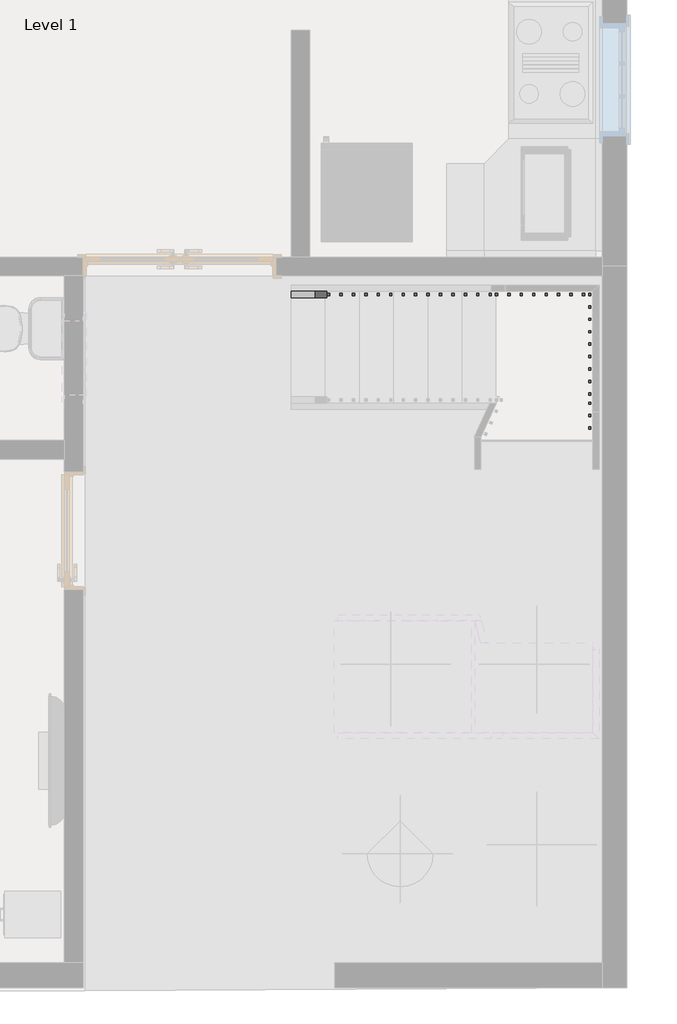
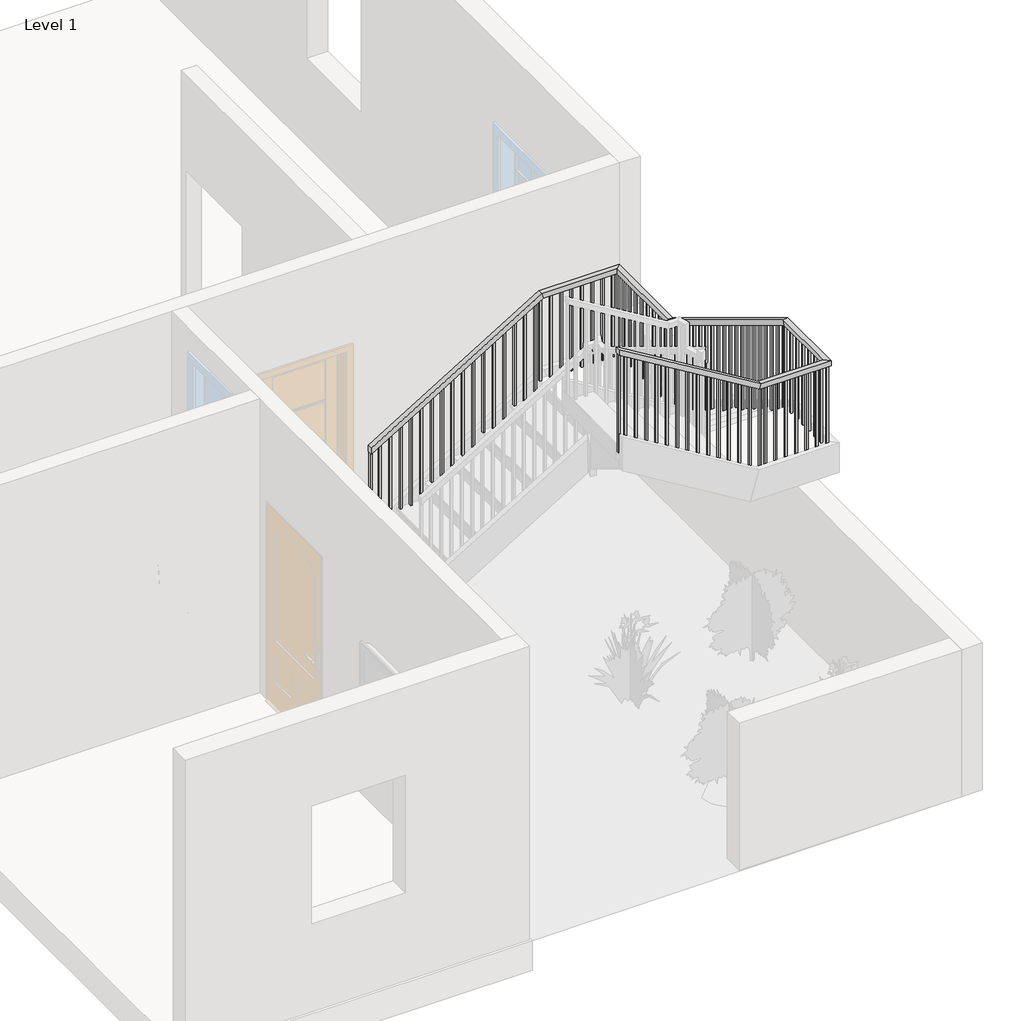
# One storey, part 3 of 4: 1 railing.
"""IFC4 building model written with IfcOpenShell, lengths in millimetres."""

from ifc_helpers import new_model, si_unit, frame, origin, place, context, project, spatial, polyline, outline, extrude, faceted_brep, element, save

model = new_model("IFC4")

# Units and contexts
model_context = context("Model", 3, world=origin())
ifc_project = project(units=[si_unit("LENGTHUNIT", "METRE", prefix="MILLI")], contexts=[model_context])

# Site, building, storey
site = spatial("IfcSite", under=ifc_project)
building = spatial("IfcBuilding", under=site)
storey = spatial("IfcBuildingStorey", under=building, Name="Level 1", Elevation=0.0)

# Railing
placement = place(None, origin())
element("IfcRailing", 1, ObjectType="Handrail - Rectangular", at=placement, inside=storey, context=model_context, shape_type="SolidModel", body=[
    faceted_brep([(-9231.9118598, 5254.5368529, 1083.7333333), (-9231.9118598, 5254.5368529, 1024.3318731), (-9231.9118598, 5203.7368529, 1024.3318731), (-9231.9118598, 5203.7368529, 1083.7333333), (-7555.5118598, 5254.5368529, 2099.7333333), (-7541.3194504, 5254.5368529, 2048.9333333), (-7541.3194504, 5203.7368529, 2048.9333333), (-7555.5118598, 5203.7368529, 2099.7333333), (-6768.1118598, 5254.5368529, 2099.7333333), (-6768.1118598, 5254.5368529, 2048.9333333), (-6818.9118598, 5203.7368529, 2048.9333333), (-6818.9118598, 5203.7368529, 2099.7333333), (-6768.1118598, 4340.1368529, 2099.7333333), (-6768.1118598, 4325.9444434, 2048.9333333), (-6818.9118598, 4325.9444434, 2048.9333333), (-6818.9118598, 4340.1368529, 2099.7333333), (-6768.1118598, 2384.3368529, 3285.0666667), (-6768.1118598, 2370.1444434, 3234.2666667), (-6818.9118598, 2370.1444434, 3234.2666667), (-6818.9118598, 2384.3368529, 3285.0666667), (-6768.1118598, 1647.7368529, 3285.0666667), (-6768.1118598, 1647.7368529, 3234.2666667), (-6818.9118598, 1698.5368529, 3234.2666667), (-6818.9118598, 1698.5368529, 3285.0666667), (-7453.9118598, 1647.7368529, 3285.0666667), (-7468.1042692, 1647.7368529, 3234.2666667), (-7468.1042692, 1698.5368529, 3234.2666667), (-7453.9118598, 1698.5368529, 3285.0666667), (-8850.9118598, 1647.7368529, 4131.7333333), (-8850.9118598, 1698.5368529, 4131.7333333), (-8850.9118598, 1698.5368529, 4072.3318731), (-8850.9118598, 1647.7368529, 4072.3318731)], [[[0, 1, 2, 3]], [[1, 0, 4, 5]], [[2, 1, 5, 6]], [[3, 2, 6, 7]], [[0, 3, 7, 4]], [[5, 4, 8, 9]], [[6, 5, 9, 10]], [[7, 6, 10, 11]], [[4, 7, 11, 8]], [[9, 8, 12, 13]], [[10, 9, 13, 14]], [[11, 10, 14, 15]], [[8, 11, 15, 12]], [[13, 12, 16, 17]], [[14, 13, 17, 18]], [[15, 14, 18, 19]], [[12, 15, 19, 16]], [[17, 16, 20, 21]], [[18, 17, 21, 22]], [[19, 18, 22, 23]], [[16, 19, 23, 20]], [[21, 20, 24, 25]], [[22, 21, 25, 26]], [[23, 22, 26, 27]], [[20, 23, 27, 24]], [[28, 29, 30, 31]], [[25, 24, 28, 31]], [[26, 25, 31, 30]], [[27, 26, 30, 29]], [[24, 27, 29, 28]]]),
    extrude(outline(polyline([(4031.9227822, -8784.2368598), (3048.0, -8784.2368598), (3048.0, -8765.1868598), (4020.3773276, -8765.1868598), (4031.9227822, -8784.2368598)])), frame((0.0, 1663.6118529, 0.0), z_axis=(0.0, 1.0, 0.0), x_axis=(0.0, 0.0, 1.0)), (0.0, 0.0, 1.0), 19.05),
    extrude(outline(polyline([(3970.3470246, -8682.6368598), (3048.0, -8682.6368598), (3048.0, -8663.5868598), (3958.80157, -8663.5868598), (3970.3470246, -8682.6368598)])), frame((0.0, 1663.6118529, 0.0), z_axis=(0.0, 1.0, 0.0), x_axis=(0.0, 0.0, 1.0)), (0.0, 0.0, 1.0), 19.05),
    extrude(outline(polyline([(3908.771267, -8581.0368598), (3048.0, -8581.0368598), (3048.0, -8561.9868598), (3897.2258125, -8561.9868598), (3908.771267, -8581.0368598)])), frame((0.0, 1663.6118529, 0.0), z_axis=(0.0, 1.0, 0.0), x_axis=(0.0, 0.0, 1.0)), (0.0, 0.0, 1.0), 19.05),
    extrude(outline(polyline([(3847.1955094, -8479.4368598), (2878.6666667, -8479.4368598), (2878.6666667, -8460.3868598), (3835.6500549, -8460.3868598), (3847.1955094, -8479.4368598)])), frame((0.0, 1663.6118529, 0.0), z_axis=(0.0, 1.0, 0.0), x_axis=(0.0, 0.0, 1.0)), (0.0, 0.0, 1.0), 19.05),
    extrude(outline(polyline([(3785.6197519, -8377.8368598), (2878.6666667, -8377.8368598), (2878.6666667, -8358.7868598), (3774.0742973, -8358.7868598), (3785.6197519, -8377.8368598)])), frame((0.0, 1663.6118529, 0.0), z_axis=(0.0, 1.0, 0.0), x_axis=(0.0, 0.0, 1.0)), (0.0, 0.0, 1.0), 19.05),
    extrude(outline(polyline([(3724.0439943, -8276.2368598), (2709.3333333, -8276.2368598), (2709.3333333, -8257.1868598), (3712.4985397, -8257.1868598), (3724.0439943, -8276.2368598)])), frame((0.0, 1663.6118529, 0.0), z_axis=(0.0, 1.0, 0.0), x_axis=(0.0, 0.0, 1.0)), (0.0, 0.0, 1.0), 19.05),
    extrude(outline(polyline([(3662.4682367, -8174.6368598), (2709.3333333, -8174.6368598), (2709.3333333, -8155.5868598), (3650.9227822, -8155.5868598), (3662.4682367, -8174.6368598)])), frame((0.0, 1663.6118529, 0.0), z_axis=(0.0, 1.0, 0.0), x_axis=(0.0, 0.0, 1.0)), (0.0, 0.0, 1.0), 19.05),
    extrude(outline(polyline([(3600.8924791, -8073.0368598), (2709.3333333, -8073.0368598), (2709.3333333, -8053.9868598), (3589.3470246, -8053.9868598), (3600.8924791, -8073.0368598)])), frame((0.0, 1663.6118529, 0.0), z_axis=(0.0, 1.0, 0.0), x_axis=(0.0, 0.0, 1.0)), (0.0, 0.0, 1.0), 19.05),
    extrude(outline(polyline([(3539.3167216, -7971.4368598), (2540.0, -7971.4368598), (2540.0, -7952.3868598), (3527.771267, -7952.3868598), (3539.3167216, -7971.4368598)])), frame((0.0, 1663.6118529, 0.0), z_axis=(0.0, 1.0, 0.0), x_axis=(0.0, 0.0, 1.0)), (0.0, 0.0, 1.0), 19.05),
    extrude(outline(polyline([(3477.740964, -7869.8368598), (2540.0, -7869.8368598), (2540.0, -7850.7868598), (3466.1955094, -7850.7868598), (3477.740964, -7869.8368598)])), frame((0.0, 1663.6118529, 0.0), z_axis=(0.0, 1.0, 0.0), x_axis=(0.0, 0.0, 1.0)), (0.0, 0.0, 1.0), 19.05),
    extrude(outline(polyline([(3416.1652064, -7768.2368598), (2540.0, -7768.2368598), (2540.0, -7749.1868598), (3404.6197519, -7749.1868598), (3416.1652064, -7768.2368598)])), frame((0.0, 1663.6118529, 0.0), z_axis=(0.0, 1.0, 0.0), x_axis=(0.0, 0.0, 1.0)), (0.0, 0.0, 1.0), 19.05),
    extrude(outline(polyline([(3354.5894488, -7666.6368598), (2370.6666667, -7666.6368598), (2370.6666667, -7647.5868598), (3343.0439943, -7647.5868598), (3354.5894488, -7666.6368598)])), frame((0.0, 1663.6118529, 0.0), z_axis=(0.0, 1.0, 0.0), x_axis=(0.0, 0.0, 1.0)), (0.0, 0.0, 1.0), 19.05),
    extrude(outline(polyline([(3293.0136913, -7565.0368598), (2370.6666667, -7565.0368598), (2370.6666667, -7545.9868598), (3281.4682367, -7545.9868598), (3293.0136913, -7565.0368598)])), frame((0.0, 1663.6118529, 0.0), z_axis=(0.0, 1.0, 0.0), x_axis=(0.0, 0.0, 1.0)), (0.0, 0.0, 1.0), 19.05),
    extrude(outline(polyline([(-7393.5868598, 1663.6118529), (-7412.6368598, 1663.6118529), (-7412.6368598, 1682.6618529), (-7393.5868598, 1682.6618529), (-7393.5868598, 1663.6118529)])), frame((0.0, 0.0, 2370.6666667), z_axis=(0.0, 0.0, 1.0), x_axis=(1.0, 0.0, 0.0)), (0.0, 0.0, 1.0), 863.6),
    extrude(outline(polyline([(-7291.9868598, 1663.6118529), (-7311.0368598, 1663.6118529), (-7311.0368598, 1682.6618529), (-7291.9868598, 1682.6618529), (-7291.9868598, 1663.6118529)])), frame((0.0, 0.0, 2370.6666667), z_axis=(0.0, 0.0, 1.0), x_axis=(1.0, 0.0, 0.0)), (0.0, 0.0, 1.0), 863.6),
    extrude(outline(polyline([(-7190.3868598, 1663.6118529), (-7209.4368598, 1663.6118529), (-7209.4368598, 1682.6618529), (-7190.3868598, 1682.6618529), (-7190.3868598, 1663.6118529)])), frame((0.0, 0.0, 2370.6666667), z_axis=(0.0, 0.0, 1.0), x_axis=(1.0, 0.0, 0.0)), (0.0, 0.0, 1.0), 863.6),
    extrude(outline(polyline([(-7088.7868598, 1663.6118529), (-7107.8368598, 1663.6118529), (-7107.8368598, 1682.6618529), (-7088.7868598, 1682.6618529), (-7088.7868598, 1663.6118529)])), frame((0.0, 0.0, 2370.6666667), z_axis=(0.0, 0.0, 1.0), x_axis=(1.0, 0.0, 0.0)), (0.0, 0.0, 1.0), 863.6),
    extrude(outline(polyline([(-6987.1868598, 1663.6118529), (-7006.2368598, 1663.6118529), (-7006.2368598, 1682.6618529), (-6987.1868598, 1682.6618529), (-6987.1868598, 1663.6118529)])), frame((0.0, 0.0, 2370.6666667), z_axis=(0.0, 0.0, 1.0), x_axis=(1.0, 0.0, 0.0)), (0.0, 0.0, 1.0), 863.6),
    extrude(outline(polyline([(-6885.5868598, 1663.6118529), (-6904.6368598, 1663.6118529), (-6904.6368598, 1682.6618529), (-6885.5868598, 1682.6618529), (-6885.5868598, 1663.6118529)])), frame((0.0, 0.0, 2370.6666667), z_axis=(0.0, 0.0, 1.0), x_axis=(1.0, 0.0, 0.0)), (0.0, 0.0, 1.0), 863.6),
    extrude(outline(polyline([(-6783.9868598, 1784.2618529), (-6783.9868598, 1765.2118529), (-6803.0368598, 1765.2118529), (-6803.0368598, 1784.2618529), (-6783.9868598, 1784.2618529)])), frame((0.0, 0.0, 2370.6666667), z_axis=(0.0, 0.0, 1.0), x_axis=(1.0, 0.0, 0.0)), (0.0, 0.0, 1.0), 863.6),
    extrude(outline(polyline([(-6783.9868598, 1885.8618529), (-6783.9868598, 1866.8118529), (-6803.0368598, 1866.8118529), (-6803.0368598, 1885.8618529), (-6783.9868598, 1885.8618529)])), frame((0.0, 0.0, 2370.6666667), z_axis=(0.0, 0.0, 1.0), x_axis=(1.0, 0.0, 0.0)), (0.0, 0.0, 1.0), 863.6),
    extrude(outline(polyline([(-6783.9868598, 1987.4618529), (-6783.9868598, 1968.4118529), (-6803.0368598, 1968.4118529), (-6803.0368598, 1987.4618529), (-6783.9868598, 1987.4618529)])), frame((0.0, 0.0, 2370.6666667), z_axis=(0.0, 0.0, 1.0), x_axis=(1.0, 0.0, 0.0)), (0.0, 0.0, 1.0), 863.6),
    extrude(outline(polyline([(-6783.9868598, 2089.0618529), (-6783.9868598, 2070.0118529), (-6803.0368598, 2070.0118529), (-6803.0368598, 2089.0618529), (-6783.9868598, 2089.0618529)])), frame((0.0, 0.0, 2370.6666667), z_axis=(0.0, 0.0, 1.0), x_axis=(1.0, 0.0, 0.0)), (0.0, 0.0, 1.0), 863.6),
    extrude(outline(polyline([(-6783.9868598, 2190.6618529), (-6783.9868598, 2171.6118529), (-6803.0368598, 2171.6118529), (-6803.0368598, 2190.6618529), (-6783.9868598, 2190.6618529)])), frame((0.0, 0.0, 2370.6666667), z_axis=(0.0, 0.0, 1.0), x_axis=(1.0, 0.0, 0.0)), (0.0, 0.0, 1.0), 863.6),
    extrude(outline(polyline([(-6783.9868598, 2292.2618529), (-6783.9868598, 2273.2118529), (-6803.0368598, 2273.2118529), (-6803.0368598, 2292.2618529), (-6783.9868598, 2292.2618529)])), frame((0.0, 0.0, 2370.6666667), z_axis=(0.0, 0.0, 1.0), x_axis=(1.0, 0.0, 0.0)), (0.0, 0.0, 1.0), 863.6),
    extrude(outline(polyline([(2419.2618529, 3204.4985397), (2419.2618529, 2201.3333333), (2400.2118529, 2201.3333333), (2400.2118529, 3216.0439943), (2419.2618529, 3204.4985397)])), frame((-6803.0368598, 0.0, 0.0), z_axis=(1.0, 0.0, 0.0), x_axis=(0.0, 1.0, 0.0)), (0.0, 0.0, 1.0), 19.05),
    extrude(outline(polyline([(2520.8618529, 3142.9227822), (2520.8618529, 2201.3333333), (2501.8118529, 2201.3333333), (2501.8118529, 3154.4682367), (2520.8618529, 3142.9227822)])), frame((-6803.0368598, 0.0, 0.0), z_axis=(1.0, 0.0, 0.0), x_axis=(0.0, 1.0, 0.0)), (0.0, 0.0, 1.0), 19.05),
    extrude(outline(polyline([(2622.4618529, 3081.3470246), (2622.4618529, 2201.3333333), (2603.4118529, 2201.3333333), (2603.4118529, 3092.8924791), (2622.4618529, 3081.3470246)])), frame((-6803.0368598, 0.0, 0.0), z_axis=(1.0, 0.0, 0.0), x_axis=(0.0, 1.0, 0.0)), (0.0, 0.0, 1.0), 19.05),
    extrude(outline(polyline([(2724.0618529, 3019.771267), (2724.0618529, 2032.0), (2705.0118529, 2032.0), (2705.0118529, 3031.3167216), (2724.0618529, 3019.771267)])), frame((-6803.0368598, 0.0, 0.0), z_axis=(1.0, 0.0, 0.0), x_axis=(0.0, 1.0, 0.0)), (0.0, 0.0, 1.0), 19.05),
    extrude(outline(polyline([(2825.6618529, 2958.1955094), (2825.6618529, 2032.0), (2806.6118529, 2032.0), (2806.6118529, 2969.740964), (2825.6618529, 2958.1955094)])), frame((-6803.0368598, 0.0, 0.0), z_axis=(1.0, 0.0, 0.0), x_axis=(0.0, 1.0, 0.0)), (0.0, 0.0, 1.0), 19.05),
    extrude(outline(polyline([(2927.2618529, 2896.6197519), (2927.2618529, 2032.0), (2908.2118529, 2032.0), (2908.2118529, 2908.1652064), (2927.2618529, 2896.6197519)])), frame((-6803.0368598, 0.0, 0.0), z_axis=(1.0, 0.0, 0.0), x_axis=(0.0, 1.0, 0.0)), (0.0, 0.0, 1.0), 19.05),
    extrude(outline(polyline([(3028.8618529, 2835.0439943), (3028.8618529, 1862.6666667), (3009.8118529, 1862.6666667), (3009.8118529, 2846.5894488), (3028.8618529, 2835.0439943)])), frame((-6803.0368598, 0.0, 0.0), z_axis=(1.0, 0.0, 0.0), x_axis=(0.0, 1.0, 0.0)), (0.0, 0.0, 1.0), 19.05),
    extrude(outline(polyline([(3130.4618529, 2773.4682367), (3130.4618529, 1862.6666667), (3111.4118529, 1862.6666667), (3111.4118529, 2785.0136913), (3130.4618529, 2773.4682367)])), frame((-6803.0368598, 0.0, 0.0), z_axis=(1.0, 0.0, 0.0), x_axis=(0.0, 1.0, 0.0)), (0.0, 0.0, 1.0), 19.05),
    extrude(outline(polyline([(3232.0618529, 2711.8924791), (3232.0618529, 1862.6666667), (3213.0118529, 1862.6666667), (3213.0118529, 2723.4379337), (3232.0618529, 2711.8924791)])), frame((-6803.0368598, 0.0, 0.0), z_axis=(1.0, 0.0, 0.0), x_axis=(0.0, 1.0, 0.0)), (0.0, 0.0, 1.0), 19.05),
    extrude(outline(polyline([(3333.6618529, 2650.3167216), (3333.6618529, 1693.3333333), (3314.6118529, 1693.3333333), (3314.6118529, 2661.8621761), (3333.6618529, 2650.3167216)])), frame((-6803.0368598, 0.0, 0.0), z_axis=(1.0, 0.0, 0.0), x_axis=(0.0, 1.0, 0.0)), (0.0, 0.0, 1.0), 19.05),
    extrude(outline(polyline([(3435.2618529, 2588.740964), (3435.2618529, 1693.3333333), (3416.2118529, 1693.3333333), (3416.2118529, 2600.2864185), (3435.2618529, 2588.740964)])), frame((-6803.0368598, 0.0, 0.0), z_axis=(1.0, 0.0, 0.0), x_axis=(0.0, 1.0, 0.0)), (0.0, 0.0, 1.0), 19.05),
    extrude(outline(polyline([(3536.8618529, 2527.1652064), (3536.8618529, 1524.0), (3517.8118529, 1524.0), (3517.8118529, 2538.710661), (3536.8618529, 2527.1652064)])), frame((-6803.0368598, 0.0, 0.0), z_axis=(1.0, 0.0, 0.0), x_axis=(0.0, 1.0, 0.0)), (0.0, 0.0, 1.0), 19.05),
    extrude(outline(polyline([(3638.4618529, 2465.5894488), (3638.4618529, 1524.0), (3619.4118529, 1524.0), (3619.4118529, 2477.1349034), (3638.4618529, 2465.5894488)])), frame((-6803.0368598, 0.0, 0.0), z_axis=(1.0, 0.0, 0.0), x_axis=(0.0, 1.0, 0.0)), (0.0, 0.0, 1.0), 19.05),
    extrude(outline(polyline([(3740.0618529, 2404.0136913), (3740.0618529, 1524.0), (3721.0118529, 1524.0), (3721.0118529, 2415.5591458), (3740.0618529, 2404.0136913)])), frame((-6803.0368598, 0.0, 0.0), z_axis=(1.0, 0.0, 0.0), x_axis=(0.0, 1.0, 0.0)), (0.0, 0.0, 1.0), 19.05),
    extrude(outline(polyline([(3841.6618529, 2342.4379337), (3841.6618529, 1354.6666667), (3822.6118529, 1354.6666667), (3822.6118529, 2353.9833882), (3841.6618529, 2342.4379337)])), frame((-6803.0368598, 0.0, 0.0), z_axis=(1.0, 0.0, 0.0), x_axis=(0.0, 1.0, 0.0)), (0.0, 0.0, 1.0), 19.05),
    extrude(outline(polyline([(3943.2618529, 2280.8621761), (3943.2618529, 1354.6666667), (3924.2118529, 1354.6666667), (3924.2118529, 2292.4076307), (3943.2618529, 2280.8621761)])), frame((-6803.0368598, 0.0, 0.0), z_axis=(1.0, 0.0, 0.0), x_axis=(0.0, 1.0, 0.0)), (0.0, 0.0, 1.0), 19.05),
    extrude(outline(polyline([(4044.8618529, 2219.2864185), (4044.8618529, 1354.6666667), (4025.8118529, 1354.6666667), (4025.8118529, 2230.8318731), (4044.8618529, 2219.2864185)])), frame((-6803.0368598, 0.0, 0.0), z_axis=(1.0, 0.0, 0.0), x_axis=(0.0, 1.0, 0.0)), (0.0, 0.0, 1.0), 19.05),
    extrude(outline(polyline([(4146.4618529, 2157.710661), (4146.4618529, 1185.3333333), (4127.4118529, 1185.3333333), (4127.4118529, 2169.2561155), (4146.4618529, 2157.710661)])), frame((-6803.0368598, 0.0, 0.0), z_axis=(1.0, 0.0, 0.0), x_axis=(0.0, 1.0, 0.0)), (0.0, 0.0, 1.0), 19.05),
    extrude(outline(polyline([(4248.0618529, 2096.1349034), (4248.0618529, 1185.3333333), (4229.0118529, 1185.3333333), (4229.0118529, 2107.6803579), (4248.0618529, 2096.1349034)])), frame((-6803.0368598, 0.0, 0.0), z_axis=(1.0, 0.0, 0.0), x_axis=(0.0, 1.0, 0.0)), (0.0, 0.0, 1.0), 19.05),
    extrude(outline(polyline([(-6783.9868598, 4425.8618529), (-6783.9868598, 4406.8118529), (-6803.0368598, 4406.8118529), (-6803.0368598, 4425.8618529), (-6783.9868598, 4425.8618529)])), frame((0.0, 0.0, 1185.3333333), z_axis=(0.0, 0.0, 1.0), x_axis=(1.0, 0.0, 0.0)), (0.0, 0.0, 1.0), 863.6),
    extrude(outline(polyline([(-6783.9868598, 4527.4618529), (-6783.9868598, 4508.4118529), (-6803.0368598, 4508.4118529), (-6803.0368598, 4527.4618529), (-6783.9868598, 4527.4618529)])), frame((0.0, 0.0, 1185.3333333), z_axis=(0.0, 0.0, 1.0), x_axis=(1.0, 0.0, 0.0)), (0.0, 0.0, 1.0), 863.6),
    extrude(outline(polyline([(-6783.9868598, 4629.0618529), (-6783.9868598, 4610.0118529), (-6803.0368598, 4610.0118529), (-6803.0368598, 4629.0618529), (-6783.9868598, 4629.0618529)])), frame((0.0, 0.0, 1185.3333333), z_axis=(0.0, 0.0, 1.0), x_axis=(1.0, 0.0, 0.0)), (0.0, 0.0, 1.0), 863.6),
    extrude(outline(polyline([(-6783.9868598, 4730.6618529), (-6783.9868598, 4711.6118529), (-6803.0368598, 4711.6118529), (-6803.0368598, 4730.6618529), (-6783.9868598, 4730.6618529)])), frame((0.0, 0.0, 1185.3333333), z_axis=(0.0, 0.0, 1.0), x_axis=(1.0, 0.0, 0.0)), (0.0, 0.0, 1.0), 863.6),
    extrude(outline(polyline([(-6783.9868598, 4832.2618529), (-6783.9868598, 4813.2118529), (-6803.0368598, 4813.2118529), (-6803.0368598, 4832.2618529), (-6783.9868598, 4832.2618529)])), frame((0.0, 0.0, 1185.3333333), z_axis=(0.0, 0.0, 1.0), x_axis=(1.0, 0.0, 0.0)), (0.0, 0.0, 1.0), 863.6),
    extrude(outline(polyline([(-6783.9868598, 4933.8618529), (-6783.9868598, 4914.8118529), (-6803.0368598, 4914.8118529), (-6803.0368598, 4933.8618529), (-6783.9868598, 4933.8618529)])), frame((0.0, 0.0, 1185.3333333), z_axis=(0.0, 0.0, 1.0), x_axis=(1.0, 0.0, 0.0)), (0.0, 0.0, 1.0), 863.6),
    extrude(outline(polyline([(-6783.9868598, 5035.4618529), (-6783.9868598, 5016.4118529), (-6803.0368598, 5016.4118529), (-6803.0368598, 5035.4618529), (-6783.9868598, 5035.4618529)])), frame((0.0, 0.0, 1185.3333333), z_axis=(0.0, 0.0, 1.0), x_axis=(1.0, 0.0, 0.0)), (0.0, 0.0, 1.0), 863.6),
    extrude(outline(polyline([(-6783.9868598, 5137.0618529), (-6783.9868598, 5118.0118529), (-6803.0368598, 5118.0118529), (-6803.0368598, 5137.0618529), (-6783.9868598, 5137.0618529)])), frame((0.0, 0.0, 1185.3333333), z_axis=(0.0, 0.0, 1.0), x_axis=(1.0, 0.0, 0.0)), (0.0, 0.0, 1.0), 863.6),
    extrude(outline(polyline([(-6853.8368598, 5238.6618529), (-6834.7868598, 5238.6618529), (-6834.7868598, 5219.6118529), (-6853.8368598, 5219.6118529), (-6853.8368598, 5238.6618529)])), frame((0.0, 0.0, 1185.3333333), z_axis=(0.0, 0.0, 1.0), x_axis=(1.0, 0.0, 0.0)), (0.0, 0.0, 1.0), 863.6),
    extrude(outline(polyline([(-6955.4368598, 5238.6618529), (-6936.3868598, 5238.6618529), (-6936.3868598, 5219.6118529), (-6955.4368598, 5219.6118529), (-6955.4368598, 5238.6618529)])), frame((0.0, 0.0, 1185.3333333), z_axis=(0.0, 0.0, 1.0), x_axis=(1.0, 0.0, 0.0)), (0.0, 0.0, 1.0), 863.6),
    extrude(outline(polyline([(-7057.0368598, 5238.6618529), (-7037.9868598, 5238.6618529), (-7037.9868598, 5219.6118529), (-7057.0368598, 5219.6118529), (-7057.0368598, 5238.6618529)])), frame((0.0, 0.0, 1185.3333333), z_axis=(0.0, 0.0, 1.0), x_axis=(1.0, 0.0, 0.0)), (0.0, 0.0, 1.0), 863.6),
    extrude(outline(polyline([(-7158.6368598, 5238.6618529), (-7139.5868598, 5238.6618529), (-7139.5868598, 5219.6118529), (-7158.6368598, 5219.6118529), (-7158.6368598, 5238.6618529)])), frame((0.0, 0.0, 1185.3333333), z_axis=(0.0, 0.0, 1.0), x_axis=(1.0, 0.0, 0.0)), (0.0, 0.0, 1.0), 863.6),
    extrude(outline(polyline([(-7260.2368598, 5238.6618529), (-7241.1868598, 5238.6618529), (-7241.1868598, 5219.6118529), (-7260.2368598, 5219.6118529), (-7260.2368598, 5238.6618529)])), frame((0.0, 0.0, 1185.3333333), z_axis=(0.0, 0.0, 1.0), x_axis=(1.0, 0.0, 0.0)), (0.0, 0.0, 1.0), 863.6),
    extrude(outline(polyline([(-7361.8368598, 5238.6618529), (-7342.7868598, 5238.6618529), (-7342.7868598, 5219.6118529), (-7361.8368598, 5219.6118529), (-7361.8368598, 5238.6618529)])), frame((0.0, 0.0, 1185.3333333), z_axis=(0.0, 0.0, 1.0), x_axis=(1.0, 0.0, 0.0)), (0.0, 0.0, 1.0), 863.6),
    extrude(outline(polyline([(-7463.4368598, 5238.6618529), (-7444.3868598, 5238.6618529), (-7444.3868598, 5219.6118529), (-7463.4368598, 5219.6118529), (-7463.4368598, 5238.6618529)])), frame((0.0, 0.0, 1185.3333333), z_axis=(0.0, 0.0, 1.0), x_axis=(1.0, 0.0, 0.0)), (0.0, 0.0, 1.0), 863.6),
    extrude(outline(polyline([(2003.771267, -7615.8368598), (1016.0, -7615.8368598), (1016.0, -7596.7868598), (2015.3167216, -7596.7868598), (2003.771267, -7615.8368598)])), frame((0.0, 5219.6118529, 0.0), z_axis=(0.0, 1.0, 0.0), x_axis=(0.0, 0.0, 1.0)), (0.0, 0.0, 1.0), 19.05),
    extrude(outline(polyline([(1942.1955094, -7717.4368598), (1016.0, -7717.4368598), (1016.0, -7698.3868598), (1953.740964, -7698.3868598), (1942.1955094, -7717.4368598)])), frame((0.0, 5219.6118529, 0.0), z_axis=(0.0, 1.0, 0.0), x_axis=(0.0, 0.0, 1.0)), (0.0, 0.0, 1.0), 19.05),
    extrude(outline(polyline([(1880.6197519, -7819.0368598), (1016.0, -7819.0368598), (1016.0, -7799.9868598), (1892.1652064, -7799.9868598), (1880.6197519, -7819.0368598)])), frame((0.0, 5219.6118529, 0.0), z_axis=(0.0, 1.0, 0.0), x_axis=(0.0, 0.0, 1.0)), (0.0, 0.0, 1.0), 19.05),
    extrude(outline(polyline([(1819.0439943, -7920.6368598), (846.6666667, -7920.6368598), (846.6666667, -7901.5868598), (1830.5894488, -7901.5868598), (1819.0439943, -7920.6368598)])), frame((0.0, 5219.6118529, 0.0), z_axis=(0.0, 1.0, 0.0), x_axis=(0.0, 0.0, 1.0)), (0.0, 0.0, 1.0), 19.05),
    extrude(outline(polyline([(1757.4682367, -8022.2368598), (846.6666667, -8022.2368598), (846.6666667, -8003.1868598), (1769.0136913, -8003.1868598), (1757.4682367, -8022.2368598)])), frame((0.0, 5219.6118529, 0.0), z_axis=(0.0, 1.0, 0.0), x_axis=(0.0, 0.0, 1.0)), (0.0, 0.0, 1.0), 19.05),
    extrude(outline(polyline([(1695.8924791, -8123.8368598), (846.6666667, -8123.8368598), (846.6666667, -8104.7868598), (1707.4379337, -8104.7868598), (1695.8924791, -8123.8368598)])), frame((0.0, 5219.6118529, 0.0), z_axis=(0.0, 1.0, 0.0), x_axis=(0.0, 0.0, 1.0)), (0.0, 0.0, 1.0), 19.05),
    extrude(outline(polyline([(1634.3167216, -8225.4368598), (677.3333333, -8225.4368598), (677.3333333, -8206.3868598), (1645.8621761, -8206.3868598), (1634.3167216, -8225.4368598)])), frame((0.0, 5219.6118529, 0.0), z_axis=(0.0, 1.0, 0.0), x_axis=(0.0, 0.0, 1.0)), (0.0, 0.0, 1.0), 19.05),
    extrude(outline(polyline([(1572.740964, -8327.0368598), (677.3333333, -8327.0368598), (677.3333333, -8307.9868598), (1584.2864185, -8307.9868598), (1572.740964, -8327.0368598)])), frame((0.0, 5219.6118529, 0.0), z_axis=(0.0, 1.0, 0.0), x_axis=(0.0, 0.0, 1.0)), (0.0, 0.0, 1.0), 19.05),
    extrude(outline(polyline([(1511.1652064, -8428.6368598), (508.0, -8428.6368598), (508.0, -8409.5868598), (1522.710661, -8409.5868598), (1511.1652064, -8428.6368598)])), frame((0.0, 5219.6118529, 0.0), z_axis=(0.0, 1.0, 0.0), x_axis=(0.0, 0.0, 1.0)), (0.0, 0.0, 1.0), 19.05),
    extrude(outline(polyline([(1449.5894488, -8530.2368598), (508.0, -8530.2368598), (508.0, -8511.1868598), (1461.1349034, -8511.1868598), (1449.5894488, -8530.2368598)])), frame((0.0, 5219.6118529, 0.0), z_axis=(0.0, 1.0, 0.0), x_axis=(0.0, 0.0, 1.0)), (0.0, 0.0, 1.0), 19.05),
    extrude(outline(polyline([(1388.0136913, -8631.8368598), (508.0, -8631.8368598), (508.0, -8612.7868598), (1399.5591458, -8612.7868598), (1388.0136913, -8631.8368598)])), frame((0.0, 5219.6118529, 0.0), z_axis=(0.0, 1.0, 0.0), x_axis=(0.0, 0.0, 1.0)), (0.0, 0.0, 1.0), 19.05),
    extrude(outline(polyline([(1326.4379337, -8733.4368598), (338.6666667, -8733.4368598), (338.6666667, -8714.3868598), (1337.9833882, -8714.3868598), (1326.4379337, -8733.4368598)])), frame((0.0, 5219.6118529, 0.0), z_axis=(0.0, 1.0, 0.0), x_axis=(0.0, 0.0, 1.0)), (0.0, 0.0, 1.0), 19.05),
    extrude(outline(polyline([(1264.8621761, -8835.0368598), (338.6666667, -8835.0368598), (338.6666667, -8815.9868598), (1276.4076307, -8815.9868598), (1264.8621761, -8835.0368598)])), frame((0.0, 5219.6118529, 0.0), z_axis=(0.0, 1.0, 0.0), x_axis=(0.0, 0.0, 1.0)), (0.0, 0.0, 1.0), 19.05),
    extrude(outline(polyline([(1203.2864185, -8936.6368598), (338.6666667, -8936.6368598), (338.6666667, -8917.5868598), (1214.8318731, -8917.5868598), (1203.2864185, -8936.6368598)])), frame((0.0, 5219.6118529, 0.0), z_axis=(0.0, 1.0, 0.0), x_axis=(0.0, 0.0, 1.0)), (0.0, 0.0, 1.0), 19.05),
    extrude(outline(polyline([(1141.710661, -9038.2368598), (169.3333333, -9038.2368598), (169.3333333, -9019.1868598), (1153.2561155, -9019.1868598), (1141.710661, -9038.2368598)])), frame((0.0, 5219.6118529, 0.0), z_axis=(0.0, 1.0, 0.0), x_axis=(0.0, 0.0, 1.0)), (0.0, 0.0, 1.0), 19.05),
    extrude(outline(polyline([(1080.1349034, -9139.8368598), (169.3333333, -9139.8368598), (169.3333333, -9120.7868598), (1091.6803579, -9120.7868598), (1080.1349034, -9139.8368598)])), frame((0.0, 5219.6118529, 0.0), z_axis=(0.0, 1.0, 0.0), x_axis=(0.0, 0.0, 1.0)), (0.0, 0.0, 1.0), 19.05),
    extrude(outline(polyline([(-7444.3868598, 1663.6118529), (-7463.4368598, 1663.6118529), (-7463.4368598, 1682.6618529), (-7444.3868598, 1682.6618529), (-7444.3868598, 1663.6118529)])), frame((0.0, 0.0, 2370.6666667), z_axis=(0.0, 0.0, 1.0), x_axis=(1.0, 0.0, 0.0)), (0.0, 0.0, 1.0), 863.6),
    extrude(outline(polyline([(-6783.9868598, 1682.6618529), (-6783.9868598, 1663.6118529), (-6803.0368598, 1663.6118529), (-6803.0368598, 1682.6618529), (-6783.9868598, 1682.6618529)])), frame((0.0, 0.0, 2370.6666667), z_axis=(0.0, 0.0, 1.0), x_axis=(1.0, 0.0, 0.0)), (0.0, 0.0, 1.0), 863.6),
    extrude(outline(polyline([(-6783.9868598, 2393.8618529), (-6783.9868598, 2374.8118529), (-6803.0368598, 2374.8118529), (-6803.0368598, 2393.8618529), (-6783.9868598, 2393.8618529)])), frame((0.0, 0.0, 2370.6666667), z_axis=(0.0, 0.0, 1.0), x_axis=(1.0, 0.0, 0.0)), (0.0, 0.0, 1.0), 863.6),
    extrude(outline(polyline([(-6783.9868598, 4349.6618529), (-6783.9868598, 4330.6118529), (-6803.0368598, 4330.6118529), (-6803.0368598, 4349.6618529), (-6783.9868598, 4349.6618529)])), frame((0.0, 0.0, 1185.3333333), z_axis=(0.0, 0.0, 1.0), x_axis=(1.0, 0.0, 0.0)), (0.0, 0.0, 1.0), 863.6),
    extrude(outline(polyline([(-6803.0368598, 5238.6618529), (-6783.9868598, 5238.6618529), (-6783.9868598, 5219.6118529), (-6803.0368598, 5219.6118529), (-6803.0368598, 5238.6618529)])), frame((0.0, 0.0, 1185.3333333), z_axis=(0.0, 0.0, 1.0), x_axis=(1.0, 0.0, 0.0)), (0.0, 0.0, 1.0), 863.6),
    extrude(outline(polyline([(-7565.0368598, 5238.6618529), (-7545.9868598, 5238.6618529), (-7545.9868598, 5219.6118529), (-7565.0368598, 5219.6118529), (-7565.0368598, 5238.6618529)])), frame((0.0, 0.0, 1185.3333333), z_axis=(0.0, 0.0, 1.0), x_axis=(1.0, 0.0, 0.0)), (0.0, 0.0, 1.0), 863.6),
    extrude(outline(polyline([(4072.3318731, -8850.9118598), (3048.0, -8850.9118598), (3048.0, -8831.8618598), (4060.7864185, -8831.8618598), (4072.3318731, -8850.9118598)])), frame((0.0, 1663.6118529, 0.0), z_axis=(0.0, 1.0, 0.0), x_axis=(0.0, 0.0, 1.0)), (0.0, 0.0, 1.0), 19.05),
    extrude(outline(polyline([(1024.3318731, -9231.9118598), (169.3333333, -9231.9118598), (169.3333333, -9212.8618598), (1035.8773276, -9212.8618598), (1024.3318731, -9231.9118598)])), frame((0.0, 5219.6118529, 0.0), z_axis=(0.0, 1.0, 0.0), x_axis=(0.0, 0.0, 1.0)), (0.0, 0.0, 1.0), 19.05),
])

save(model, "model.ifc")

# Revit data of these elements
# Type "Handrail - Rectangular"
#   Assembly Code = "C2010400"
#   built-in parameter 1008612 = 0.0416667 (stored number, unit not read)
#   built-in parameter 1008611 = 0.0416667 (stored number, unit not read)
#   built-in parameter 1008609 = 0.333333 (stored number, unit not read)
#   built-in parameter 1008604 = 0.166667 (stored number, unit not read)
#   built-in parameter 1008603 = 0.166667 (stored number, unit not read)
#   Railing Height = 3' - 0"
#   built-in parameter 1008630 = 2
#   built-in parameter 1008610 = 2
#   built-in parameter 1008618 = Baluster - Square : 3/4"
# Element 1 (IfcRailing, "Handrail - Rectangular")
#   Phase Created = New Construction
